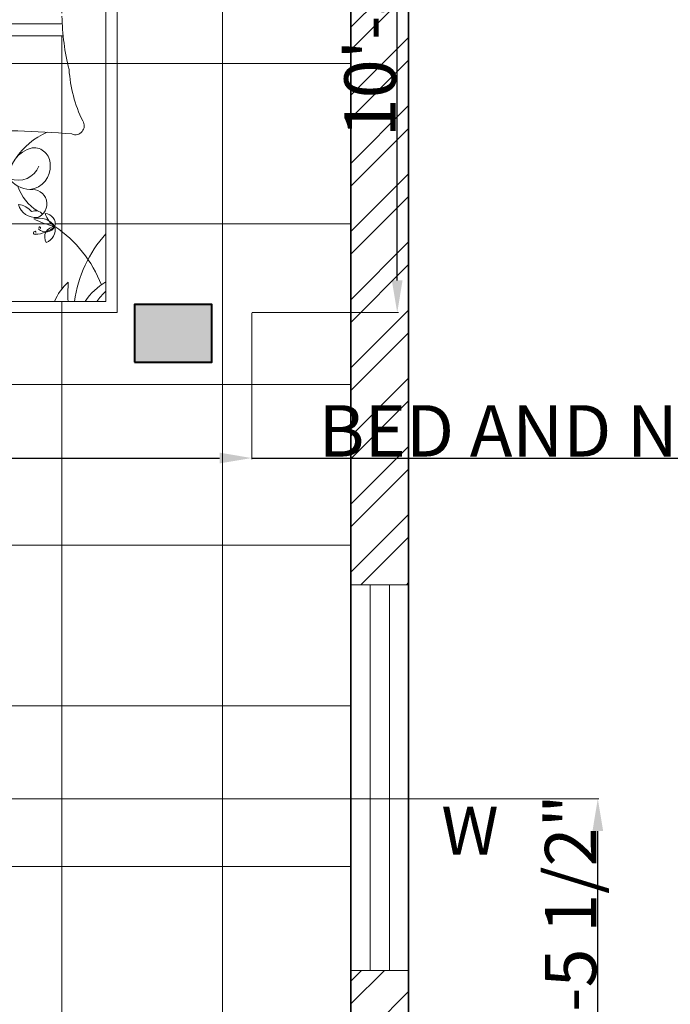
# Model space of a CAD drawing. Units: inches. Extents: x 351 to 1738, y -265 to 286.
# Tile 35 of 38: x 1506 to 1607, y -35 to 118. Entities that reach past the tile are written whole.
import ezdxf

# ---------------------------------------------------------------- set-up
doc = ezdxf.new("R2010")
doc.units = ezdxf.units.IN
doc.header["$MEASUREMENT"] = 0
for name, color, linetype, lineweight in [('A-ANNO-DIMS', 2, 'Continuous', 18), ('A-ANNO-SYMB', 7, 'Continuous', 18), ('A-COLS', 7, 'Continuous', 40), ('A-COLS-PATT', 6, 'Continuous', 13), ('A-FLOR-PATT', 9, 'Continuous', 9), ('A-FURN', 18, 'Continuous', 13), ('A-GLAZ', 4, 'Continuous', 18), ('A-WALL', 7, 'Continuous', 35), ('A-WALL-PATT', 152, 'Continuous', 13)]:
    doc.layers.add(name, color=color, linetype=linetype, lineweight=lineweight)
doc.styles.add('Annotative', font='arial.ttf')
doc.styles.get("Standard").update_dxf_attribs({"font": 'arial.ttf'})
doc.dimstyles.get("Standard").update_dxf_attribs({"dimtxt": 8, "dimasz": 5, "dimexe": 0.18, "dimexo": 0.0625, "dimgap": 0.09, "dimtad": 1, "dimtoh": 1, "dimzin": 0, "dimdsep": 46, "dimlunit": 4, "dimtxsty": 'Standard', "dimcen": 0, "dimclre": 256, "dimadec": 0, "dimazin": 0, "dimtfac": 1, "dimtofl": 0, "dimtmove": 0, "dimatfit": 3, "dimfxl": 1, "dimtolj": 1, "dimtzin": 0, "dimlwe": -1, "dimarcsym": 0})

# ---------------------------------------------------------------- blocks, each defined once
blk = doc.blocks.new('BED-DOUBLE-W-NIGHTSTANDS')
for p, q in [((121.41, 44.95), (28.44, 44.95)), ((121.55, 43.07), (28.44, 43.07))]:
    blk.add_line(p, q)
for points in [[(121.56, 54.36), (129.93, 54.36), (129.93, 0), (19.92, 0), (19.92, 54.36), (28.45, 54.36)], [(28.45, 52.61), (21.67, 52.61), (21.67, 1.75), (128.18, 1.75), (128.18, 52.61), (121.53, 52.61)]]:
    blk.add_lwpolyline(points)
blk.add_lwpolyline([(121.36, 46.14, 0.056112), (122.46, 37.83, 0.095341), (124.58, 29.84)], format="xyb")
for centre, radius, start, end in [((123.44, 29.07), 1.38, 246.5219, 33.8264), ((110.71, -118.52), 146.84, 85.2402, 91.8035), ((123.63, 17.62), 11.42, 113.6453, 146.3329), ((117.76, 21.21), 4.54, 103.079, 184.7067), ((116.98, 23.1), 2.55, 358.9462, 95.5144), ((115.93, 22.74), 3.61, 277.1143, 5.0551), ((114.52, 24.1), 3.5, 248.5779, 338.4181), ((116.56, 23.54), 4.38, 215.9599, 267.6409), ((121.25, 21.91), 7.12, 198.2955, 238.7386), ((116.76, 16.92), 2.26, 289.1312, 99.736), ((117.31, 17.61), 2.83, 195.6955, 274.031), ((114.26, 13.85), 3.01, 38.4175, 83.8338), ((117.23, 14.47), 1.39, 36.7319, 116.0245), ((122.02, 16.28), 3.37, 194.7031, 238.6173), ((118.68, 13.79), 1.63, 346.272, 87.0484), ((117.74, 11.59), 3.12, 35.7657, 104.5347), ((123.26, 26.86), 13.79, 242.8176, 257.4827), ((117.16, 12.42), 0.245, 78.5166, 272.0648), ((116.99, 17.16), 4.98, 272.0648, 311.1598), ((117.18, 12.55), 0.119, 322.0591, 78.5166), ((118.84, 14.16), 1.61, 226.2238, 332.3173), ((117.9, 13.23), 0.128, 290.2667, 226.2271), ((120.32, 11.76), 1.65, 91.7131, 211.5367), ((118.13, 12.94), 2.19, 290.9613, 12.2885), ((109.14, -2.86), 19.71, 21.4092, 55.6135), ((142.85, -0.91), 19.71, 138.1144, 172.255), ((127.59, -1.32), 8.01, 131.0454, 157.4453), ((149.54, 2.98), 27.26, 176.3481, 182.5919), ((132.97, -3.55), 9.6, 119.8884, 146.5383), ((136.42, -5.34), 11.97, 133.5186, 143.6964)]:
    blk.add_arc(centre, radius, start, end)
blk = doc.blocks.new('COL-9x12')
blk.add_lwpolyline([(0, 12), (0, 0), (9, 0), (9, 12)], close=True)
blk = doc.blocks.new('WIN-60')
for p, q in [((0, 6), (60, 6)), ((0, 3), (60, 3))]:
    blk.add_line(p, q)
blk.add_lwpolyline([(60, 0), (60, 9), (0, 9), (0, 0)], close=True)
blk = doc.blocks.new('*D46')
at = {"layer": 'A-ANNO-DIMS', "transparency": 16777216}
for p, q in [((1391.39, 72.13), (1391.39, 49.37)), ((1542.29, 72.13), (1542.29, 49.37))]:
    blk.add_line(p, q, dxfattribs=at)
at = {"layer": 'A-ANNO-DIMS', "color": 0, "lineweight": -2, "transparency": 16777216}
for p, q in [((1396.39, 49.55), (1537.29, 49.55)), ((1542.29, 49.55), (1738.09, 49.55))]:
    blk.add_line(p, q, dxfattribs=at)
at = {"layer": 'A-ANNO-DIMS', "color": 0, "transparency": 16777216}
for points in [[(1396.39, 50.39), (1396.39, 48.72), (1391.39, 49.55)], [(1537.29, 50.39), (1537.29, 48.72), (1542.29, 49.55)]]:
    blk.add_solid(points, dxfattribs=at)
at = {"layer": 'Defpoints', "color": 0, "transparency": 16777216}
for p in [(1391.39, 72.19), (1542.29, 72.19), (1542.29, 49.55)]:
    blk.add_point(p, dxfattribs=at)
at = {"layer": 'A-ANNO-DIMS', "color": 0, "transparency": 16777216, "insert": (1642.69, 53.78), "char_height": 8, "attachment_point": 5}
blk.add_mtext('\\A1;BED AND NIGHTSTANDS 12\'-7" TYP.', dxfattribs=at)
blk = doc.blocks.new('*D47')
at = {"layer": 'A-ANNO-DIMS', "transparency": 16777216}
for p, q in [((1542.36, 200.52), (1565.11, 200.52)), ((1542.36, 72.19), (1565.11, 72.19))]:
    blk.add_line(p, q, dxfattribs=at)
at = {"layer": 'A-ANNO-DIMS', "color": 0, "lineweight": -2, "transparency": 16777216}
blk.add_line((1564.93, 77.19), (1564.93, 195.52), dxfattribs=at)
at = {"layer": 'A-ANNO-DIMS', "color": 0, "transparency": 16777216}
for points in [[(1564.1, 195.52), (1565.76, 195.52), (1564.93, 200.52)], [(1564.1, 77.19), (1565.76, 77.19), (1564.93, 72.19)]]:
    blk.add_solid(points, dxfattribs=at)
at = {"layer": 'Defpoints', "color": 0, "transparency": 16777216}
for p in [(1542.29, 200.52), (1564.93, 200.52), (1542.29, 72.19)]:
    blk.add_point(p, dxfattribs=at)
at = {"layer": 'A-ANNO-DIMS', "color": 0, "transparency": 16777216, "insert": (1560.7, 136.35), "char_height": 8, "attachment_point": 5, "rotation": 90}
blk.add_mtext('\\A1;10\'-8 1/2" TYP.', dxfattribs=at)
blk = doc.blocks.new('*D66')
at = {"layer": 'A-ANNO-DIMS', "transparency": 16777216}
for p, q in [((1384.27, -3.5), (1596.33, -3.5)), ((1384.27, -45), (1596.33, -45))]:
    blk.add_line(p, q, dxfattribs=at)
at = {"layer": 'A-ANNO-DIMS', "color": 0, "lineweight": -2, "transparency": 16777216}
blk.add_line((1596.15, -40), (1596.15, -8.5), dxfattribs=at)
at = {"layer": 'A-ANNO-DIMS', "color": 0, "transparency": 16777216}
for points in [[(1595.32, -8.5), (1596.99, -8.5), (1596.15, -3.5)], [(1595.32, -40), (1596.99, -40), (1596.15, -45)]]:
    blk.add_solid(points, dxfattribs=at)
at = {"layer": 'Defpoints', "color": 0, "transparency": 16777216}
for p in [(1384.2, -3.5), (1596.15, -3.5), (1384.2, -45)]:
    blk.add_point(p, dxfattribs=at)
at = {"layer": 'A-ANNO-DIMS', "color": 0, "transparency": 16777216, "insert": (1591.92, -24.25), "char_height": 8, "attachment_point": 5, "rotation": 90}
blk.add_mtext('\\A1;3\'-5 1/2"', dxfattribs=at)

msp = doc.modelspace()

# ---------------------------------------------------------------- hatches: boundary and pattern name
at = {"layer": 'A-COLS-PATT'}
h = msp.add_hatch(color=256, dxfattribs=at)
h.dxf.hatch_style = 1
h.paths.add_polyline_path([(1112.704, 237.963), (1103.704, 237.963), (1103.704, 228.963), (1112.704, 228.963)])
h.paths.add_polyline_path([(1115.704, 237.963), (1112.704, 237.963), (1112.704, 228.963), (1115.704, 228.963)])
h.paths.add_polyline_path([(1043.704, 255.963), (1034.704, 255.963), (1034.704, 243.963), (1043.704, 243.963)])
h.paths.add_polyline_path([(1043.704, 210.963), (1034.704, 210.963), (1034.704, 198.963), (1043.704, 198.963)])
h.paths.add_polyline_path([(1043.704, -45.037), (1034.704, -45.037), (1034.704, -57.037), (1043.704, -57.037)])
h.paths.add_polyline_path([(1112.704, -45.037), (1103.704, -45.037), (1103.704, -57.037), (1112.704, -57.037)])
h.paths.add_polyline_path([(1112.704, -161.037), (1103.704, -161.037), (1103.704, -164.037), (1103.704, -173.037), (1112.704, -173.037)])
h.paths.add_polyline_path([(1043.704, -161.037), (1034.704, -161.037), (1034.704, -173.037), (1043.704, -173.037)])
h.paths.add_polyline_path([(1248.549, -164.037), (1236.549, -164.037), (1236.549, -173.037), (1248.549, -173.037)])
h.paths.add_polyline_path([(1248.549, -50), (1236.549, -50), (1236.549, -59), (1248.549, -59)])
h.paths.add_polyline_path([(1248.704, 73.463), (1244.704, 73.463), (1244.704, 64.463), (1248.704, 64.463)])
h.paths.add_polyline_path([(1244.704, 73.463), (1236.704, 73.463), (1236.704, 64.463), (1244.704, 64.463)])
h.paths.add_polyline_path([(1248.704, 237.963), (1236.704, 237.963), (1236.704, 228.963), (1248.704, 228.963)])
h.paths.add_polyline_path([(1392.204, 237.963), (1380.204, 237.963), (1380.204, 228.963), (1392.204, 228.963)])
h.paths.add_polyline_path([(1536.064, 237.963), (1524.064, 237.963), (1524.064, 228.963), (1536.064, 228.963)])
h.paths.add_polyline_path([(1536.064, 73.463), (1524.064, 73.463), (1524.064, 64.463), (1536.064, 64.463)])
h.paths.add_polyline_path([(1384.204, 73.463), (1380.204, 73.463), (1380.204, 64.463), (1384.204, 64.463)])
h.paths.add_polyline_path([(1392.064, 73.463), (1384.204, 73.463), (1384.204, 64.463), (1392.064, 64.463)])
h.paths.add_polyline_path([(1536.064, -53.037), (1524.064, -53.037), (1524.064, -57.037), (1536.064, -57.037)])
h.paths.add_polyline_path([(1536.064, -48.037), (1524.064, -48.037), (1524.064, -53.037), (1536.064, -53.037)])
h.paths.add_polyline_path([(1392.064, -48.037), (1380.064, -48.037), (1380.064, -56.5), (1380.065, -57.037), (1392.064, -57.037)])
h.paths.add_polyline_path([(1536.064, -164.037), (1524.064, -164.037), (1524.064, -173.037), (1536.064, -173.037)])
at = {"layer": 'A-FLOR-PATT', "transparency": 33554559}
h = msp.add_hatch(dxfattribs=at)
h.set_pattern_fill('ANSI37', color=256, scale=200, angle=135)
h.set_pattern_definition([(180, (1112.704, -164.037), (-2e-15, -25), []), (270, (1112.704, -164.037), (25, -5e-15), [])])
h.paths.add_polyline_path([(1380.064, 73.463), (1380.132, 148.463), (1338.064, 148.463), (1290.704, 148.463), (1290.704, 88.463), (1248.704, 88.463), (1248.704, -2.009), (1244.704, -2.009), (1244.704, 142.457), (1160.704, 142.457), (1160.704, 158.963), (1160.704, 170.137), (1160.704, 206.137), (1160.704, 228.963), (1112.704, 228.963), (1112.704, 209.963), (1112.704, 168.963), (1124.704, 168.963), (1124.704, 162.963), (1112.704, 162.963), (1112.704, 64.463), (1112.704, 60.463), (1112.704, 0.463), (1112.704, -48.026), (1146.804, -47.981), (1146.804, -35.691), (1207.804, -35.691), (1207.804, -47.902), (1236.542, -47.864), (1236.544, -50.009), (1248.5, -50.009), (1248.506, -102.915), (1248.512, -150.915), (1248.514, -164.037), (1248.549, -164.037), (1273.017, -164.037), (1273.017, -128.799), (1355.24, -128.799), (1355.24, -164.037), (1384.204, -164.037), (1384.204, -57.037), (1380.064, -57.037), (1380.064, -48.037), (1392.064, -48.037), (1392.064, -53.037), (1406.549, -53.037), (1406.549, -57.037), (1401.204, -57.037), (1401.204, -147.037), (1468.204, -147.037), (1468.204, -138.5), (1472.204, -138.5), (1472.204, -102.5), (1468.204, -102.5), (1468.204, -57.037), (1442.549, -57.037), (1442.549, -53.037), (1463.049, -53.037), (1463.049, -40.747), (1524.049, -40.747), (1524.049, -48.037), (1536.064, -48.037), (1536.064, -53.037), (1557.704, -53.037), (1557.704, 204.963), (1384.204, 204.963), (1384.204, 73.463), (1392.064, 73.463), (1392.064, 64.463), (1384.204, 64.463), (1384.204, -3.5), (1380.204, -3.537), (1380.204, 64.463), (1380.064, 64.463)])
h.paths.add_polyline_path([(1510.714, 86.458, -0.1039845), (1511.661, 85.595, 0.4704384), (1510.158, 87.614, 0.0961001)], flags=16)
h.paths.add_polyline_path([(1510.443, 100.266, 0.009798), (1504.693, 100.48, 0.0287898), (1504.6, 99.767, -0.1653311), (1505.519, 96.135, -0.1436014)], flags=16)
h.paths.add_polyline_path([(1487.201, 85.595, -0.1039845), (1488.148, 86.458, 0.0961001), (1488.704, 87.614, 0.4704384)], flags=0)
h.paths.add_polyline_path([(1495.052, 100.43), (1494.178, 100.43, -0.0264629), (1494.262, 99.774, -0.1442193)], flags=16)
h.paths.add_polyline_path([(1444.485, 86.458, -0.1039845), (1445.433, 85.595, 0.4704384), (1443.93, 87.614, 0.0961001)], flags=16)
h.paths.add_polyline_path([(1420.972, 85.595, -0.1039845), (1421.92, 86.458, 0.0961001), (1422.475, 87.614, 0.4704384)], flags=16)
h.paths.add_polyline_path([(1428.632, 100.335, 0.0010541), (1427.971, 100.309, -0.0215241), (1428.033, 99.774, -0.1143008)], flags=16)
h.paths.add_polyline_path([(1419.906, 143.708, 0.0249793), (1420.222, 157.526), (1421.573, 159.101), (1421.573, 175.369), (1391.393, 175.369), (1391.393, 200.519), (1542.294, 200.519), (1542.294, 175.369), (1512.028, 175.369, 0.0198653), (1511.521, 153.838, 0.0251335), (1512.758, 118.323, 0.0205529), (1512.942, 115.253), (1419.834, 115.253, -0.0004142), (1419.843, 124.798), (1413.059, 124.798), (1413.059, 84.437, -0.0618528), (1415.831, 80.45, -0.0930773), (1420.972, 85.595, -0.2675367), (1422.371, 84.732, 0.0851103), (1424.052, 84.616, -0.8853927), (1424.033, 84.851, -1.1258145), (1424.073, 84.366, -0.0879871), (1422.371, 84.732, -0.2675367), (1422.326, 83.089, -0.3705421), (1420.972, 85.595, 0.0930773), (1415.831, 80.45, -0.0874142), (1417.914, 73.937), (1418.941, 73.937, 0.0272504), (1418.913, 76.906, -0.1157032), (1421.051, 73.937), (1445.354, 73.937, -0.1157032), (1447.492, 76.906, 0.0272504), (1447.464, 73.937), (1448.491, 73.937, -0.0874142), (1450.574, 80.45, 0.0930773), (1445.433, 85.595, -0.3705421), (1444.079, 83.089, -0.2675367), (1444.034, 84.732, -0.0879871), (1442.332, 84.366, -1.1258145), (1442.372, 84.851, -2.0327363), (1442.364, 84.368, 0.0863779), (1444.034, 84.732, -0.2675367), (1445.433, 85.595, -0.0930773), (1450.574, 80.45, -0.2577317), (1466.483, 90.927, -0.4786702), (1468.832, 91.907, -0.4786702), (1471.18, 90.927, -0.26264), (1483.053, 81.78, -0.0718662), (1487.201, 85.595, -0.2675367), (1488.6, 84.732, 0.0851103), (1490.28, 84.616, -0.8853927), (1490.262, 84.851, -1.1258145), (1490.301, 84.366, -0.0879871), (1488.6, 84.732, -0.2675367), (1488.554, 83.089, -0.3705421), (1487.201, 85.595, 0.0718662), (1483.053, 81.78, -0.1320648), (1484.143, 73.937), (1485.169, 73.937, 0.0272504), (1485.142, 76.906, -0.1157032), (1487.28, 73.937), (1511.582, 73.937, -0.1157032), (1513.72, 76.906, 0.0272504), (1513.693, 73.937), (1514.719, 73.937, -0.0874142), (1516.802, 80.45, 0.0930773), (1511.661, 85.595, -0.3705421), (1510.308, 83.089, -0.2675367), (1510.262, 84.732, -0.0879871), (1508.561, 84.366, -1.1258145), (1508.601, 84.851, -2.0327363), (1508.592, 84.368, 0.0863779), (1510.262, 84.732, -0.2675367), (1511.661, 85.595, -0.0930773), (1516.802, 80.45, -0.0618528), (1519.575, 84.437), (1519.575, 73.937), (1413.059, 73.937), (1413.059, 124.798), (1419.843, 124.798, -0.0008205)], flags=16)
h.paths.add_polyline_path([(1220.149, 54.133, -0.1039845), (1220.869, 53.476, 0.4704384), (1219.727, 55.011, 0.0961001)], flags=16)
h.paths.add_polyline_path([(1219.944, 64.626, 0.009798), (1215.574, 64.789, 0.0287898), (1215.503, 64.247, -0.1653311), (1216.201, 61.487, -0.1436014)], flags=16)
h.paths.add_polyline_path([(1209.779, 64.449, 0.0974459), (1209.339, 64.751), (1208.247, 64.751, 0.1273905), (1207.7, 64.326, 0.1715858), (1206.95, 61.475, -0.1588542), (1207.636, 59.45, 0.0158984), (1207.795, 59.218, 0.0615457), (1208.598, 59.616, 0.1754158), (1208.638, 60.099, -0.2847793), (1209.348, 62.472, 0.3262165)], flags=16)
h.paths.add_polyline_path([(1169.818, 54.133, -0.1039845), (1170.538, 53.476, 0.4704384), (1169.396, 55.011, 0.0961001)], flags=16)
h.paths.add_polyline_path([(1159.017, 62.472, 0.2847642), (1158.307, 60.099, -0.1754332), (1158.267, 59.616, 0.3929302), (1159.448, 64.449, -0.3262298)], flags=16)
h.paths.add_polyline_path([(1156.342, 58.239, -0.1783213), (1154.011, 55.31, -0.1747359), (1154.722, 55.233, -0.2008015), (1156.27, 56.086, 0.1269899), (1157.283, 58.991, -0.0912053)], flags=16)
h.paths.add_polyline_path([(1156.624, 61.413, 0.1572752), (1157.316, 64.247, 0.1696217)], flags=16)
h.paths.add_polyline_path([(1152.67, 54.133, -0.0961001), (1151.95, 53.476, 0.0640762), (1154.465, 54.384, 0.1990158)], flags=16)
h.paths.add_polyline_path([(1202.281, 53.476, -0.1039845), (1203, 54.133, 0.0961001), (1203.423, 55.011, 0.4704384)], flags=0)
h.paths.add_polyline_path([(1151.139, 97.64, 0.0249793), (1151.379, 108.141), (1152.406, 109.338), (1152.406, 121.701), (1129.47, 121.701), (1129.47, 140.814), (1244.149, 140.814), (1244.149, 121.701), (1221.148, 121.701, 0.0198653), (1220.763, 105.338, 0.0251335), (1221.703, 78.349, 0.0205529), (1221.843, 76.016), (1151.078, 76.016, -0.1287433), (1148.786, 65.037, 0.5393525), (1150.327, 64.171, -0.027594), (1163.481, 64.751, 0.0976954), (1163.04, 64.449, 0.3262165), (1163.471, 62.472, -0.2847765), (1164.181, 60.099, -0.1947567), (1165.846, 61.443, -0.1554021), (1165.172, 64.247, -0.1660224), (1165.869, 61.475, -0.1770142), (1167.852, 62.77, -0.4482027), (1169.974, 60.807, -0.3934987), (1167.679, 57.86, -0.8955483), (1168.438, 54.524, -0.3557668), (1166.218, 56.086, -0.066024), (1165.505, 57.539), (1165.251, 56.243, -0.3717324), (1164.02, 59.758, -0.3736141), (1163.04, 64.449, -0.0976954), (1163.481, 64.751, 0.0213538), (1153.294, 64.429, -0.1341826), (1156.695, 61.368, 0.1868727), (1154.636, 62.77, 0.4482027), (1152.514, 60.807, 0.4037263), (1154.905, 57.846, 0.7112192), (1153.334, 55, 0.5315397), (1151.95, 53.476, -0.2675367), (1153.013, 52.821, 0.0851103), (1154.29, 52.732, -0.8853927), (1154.276, 52.911, -1.1258145), (1154.306, 52.543, -0.0879871), (1153.013, 52.821, -0.2675367), (1152.978, 51.572, -0.3705421), (1151.95, 53.476, 0.0930773), (1148.043, 49.566, -0.0874142), (1149.626, 44.617), (1150.406, 44.617, 0.0272504), (1150.385, 46.873, -0.1157032), (1152.01, 44.617), (1170.478, 44.617, -0.1157032), (1172.103, 46.873, 0.0272504), (1172.082, 44.617), (1172.862, 44.617, -0.0874142), (1174.445, 49.566, 0.0930773), (1170.538, 53.476, -0.3705421), (1169.51, 51.572, -0.2675367), (1169.475, 52.821, -0.0879871), (1168.182, 52.543, -1.1258145), (1168.212, 52.911, -2.0327363), (1168.206, 52.544, 0.0863779), (1169.475, 52.821, -0.2675367), (1170.538, 53.476, -0.0930773), (1174.445, 49.566, -0.2577317), (1186.536, 57.528, -0.4786702), (1188.321, 58.273, -0.4786702), (1190.106, 57.528, -0.26264), (1199.128, 50.577, -0.0718662), (1202.281, 53.476, -0.2675367), (1203.344, 52.821, 0.0851103), (1204.621, 52.732, -0.8853927), (1204.607, 52.911, -1.1258145), (1204.637, 52.543, -0.0879871), (1203.344, 52.821, -0.2675367), (1203.309, 51.572, -0.3705421), (1202.281, 53.476, 0.0718662), (1199.128, 50.577, -0.1320648), (1199.957, 44.617), (1200.737, 44.617, 0.0272504), (1200.716, 46.873, -0.1157032), (1202.341, 44.617), (1220.809, 44.617, -0.1157032), (1222.434, 46.873, 0.0272504), (1222.413, 44.617), (1223.193, 44.617, -0.0874142), (1224.776, 49.566, 0.0930773), (1220.869, 53.476, -0.3705421), (1219.841, 51.572, -0.2675367), (1219.806, 52.821, -0.0879871), (1218.513, 52.543, -1.1258145), (1218.543, 52.911, -2.0327363), (1218.537, 52.544, 0.0863779), (1219.806, 52.821, -0.2675367), (1220.869, 53.476, -0.0930773), (1224.776, 49.566, -0.0618528), (1226.883, 52.597), (1226.883, 44.617), (1145.936, 44.617), (1145.936, 83.269), (1151.091, 83.269, -0.0008205)], flags=16)
h.paths.add_polyline_path([(1218.01, 57.86, -0.8955483), (1218.769, 54.524, -0.3557668), (1216.549, 56.086, -0.066024), (1215.836, 57.539), (1215.582, 56.243, -0.3717324), (1214.351, 59.758, -0.3736141), (1213.371, 64.449, 0.3262165), (1213.802, 62.472, -0.2847765), (1214.512, 60.099, -0.1947567), (1216.177, 61.443, -0.1799907), (1218.183, 62.77, -0.4482027), (1220.305, 60.807, -0.3934987)], flags=16)
h.paths.add_polyline_path([(1424.735, 91.363, -0.3934987), (1421.715, 95.241, -0.4482027), (1424.507, 97.824, -0.1799907), (1427.147, 96.077, -0.1947567), (1429.338, 94.309, -0.2847765), (1430.272, 97.432, 0.3262165), (1430.839, 100.034, -0.3736141), (1429.55, 93.861, -0.3717324), (1427.929, 89.235), (1427.596, 90.941, -0.066024), (1426.657, 89.029, -0.3557668), (1423.736, 86.973, -0.8955483)], flags=16)
h.paths.add_polyline_path([(1238.033, 131.257, -1), (1227.329, 131.257, -1)], flags=0)
h.paths.add_polyline_path([(1235.357, 131.257, -1), (1230.005, 131.257, -1)], flags=0)
h.paths.add_polyline_path([(1214.039, 54.243, 0.1543819), (1214.38, 53.992, 0.3589549), (1213.613, 54.016, 0.6039484), (1214.379, 53.657, 0.3713191), (1213.968, 52.872, 0.1879935), (1214.312, 52.809, -0.592455), (1213.953, 52.967, -0.2942791), (1214.083, 53.691, -1.3001871), (1213.881, 54.134, -0.2837621), (1214.469, 53.896, 1.1509396)], flags=16)
h.paths.add_polyline_path([(1212.091, 56.286, -0.4084338), (1211.337, 56.445, -0.0362594), (1211.098, 56.848, -0.2360976), (1211.59, 56.63, 0.0353445), (1211.835, 56.543, -0.4752408), (1212.091, 56.286, -0.4752408), (1212.438, 56.182, 0.0353445), (1212.631, 56.007, -0.2360976), (1213.056, 55.676, -0.0362594), (1212.588, 55.697, -0.4084338)], flags=16)
h.paths.add_polyline_path([(1211.469, 50.297, 0.296043), (1210.47, 50.527, 0.310883), (1211.931, 50.148, 0.0212546)], flags=16)
h.paths.add_polyline_path([(1213.739, 51.818, -0.0362594), (1213.271, 51.838, -0.4084337), (1212.774, 52.427, -0.0947856), (1212.293, 50.703, 1.1504738), (1212.911, 50.232, 0.1662877), (1213.265, 50.68, -0.0252543), (1212.603, 50.13, 1.0879317), (1212.471, 49.407, 0.1662877), (1213.02, 49.251, -0.016128), (1212.567, 49.563, -0.286859), (1212.217, 49.638, 0.0221563), (1212.046, 50.055, -0.6461302), (1212.185, 50.498, 0.0884116), (1212.732, 52.077, -1.1860374), (1213.121, 52.323, 0.0353445), (1213.314, 52.148, -0.2360976)], flags=16)
h.paths.add_polyline_path([(1212.094, 50.342, -0.0485241), (1211.54, 49.605, -1.1038339), (1211.397, 48.738, -0.7855147), (1211.683, 48.254, -0.3920429), (1210.948, 48.525, -0.3928194), (1210.561, 47.995, -0.592455), (1210.201, 48.153, -0.2942791), (1210.331, 48.877, -0.7041716), (1210.316, 49.592, -0.6793441), (1210.729, 50.112, 0.5636764)], flags=16)
h.paths.add_polyline_path([(1211.274, 49.829, -0.1398258), (1210.745, 49.859, -0.2178785), (1210.948, 49.509, -0.4985724)], flags=0)
h.paths.add_polyline_path([(1433.426, 81.49, -0.181571), (1434.245, 81.788, -0.0080665), (1433.726, 82.205, 0.0455784), (1432.755, 81.242, 0.1790113)], flags=16)
h.paths.add_polyline_path([(1434.146, 81.009, -0.1324418), (1433.645, 80.771, 0.2590893), (1433.234, 80.471, -0.1802109), (1433.392, 80.805, -0.1699398), (1432.758, 81.109, 0.0326525), (1433.273, 80.474, -0.4933627), (1434.046, 80.146, -0.3904966)], flags=16)
h.paths.add_polyline_path([(1434.83, 80.047, -0.9475376), (1435.294, 79.576, -0.2991282), (1434.625, 79.404, -0.2704392), (1435.01, 78.591, -0.592455), (1434.537, 78.382, -0.3928194), (1434.027, 79.08, -0.3920429), (1433.06, 78.723, -0.3520423), (1433.003, 79.197, -0.1972159), (1433.75, 79.734, -0.7136405), (1434.447, 79.939, -0.2147903), (1434.819, 80.475, 0.4088333), (1435.075, 80.803, -0.2261519)], flags=16)
h.paths.add_polyline_path([(1432.67, 81.217, -0.4542182), (1431.897, 79.923, -0.4144105), (1431.301, 80.035, 0.0161291), (1431.897, 80.445, 0.2795702), (1432.073, 80.871, -0.2895037), (1431.103, 81.321, -0.4144105), (1430.978, 81.915, 0.0161296), (1431.586, 81.521, 0.341293), (1432.125, 81.583, -0.8131856)], flags=16)
h.paths.add_polyline_path([(1429.893, 86.381, -0.9475376), (1430.358, 85.91, -0.1731062), (1429.984, 85.712, -0.0388172), (1431.625, 84.214, -0.0879005), (1432.097, 88.549, -0.0497684), (1431.254, 88.49, -0.2360976), (1431.814, 88.925, 0.0353445), (1432.067, 89.155, -0.4752408), (1432.524, 89.291, -0.4752408), (1432.86, 89.63, 0.0353445), (1433.182, 89.744, -0.2360976), (1433.83, 90.032, -0.0362594), (1433.516, 89.502, -0.4084338), (1432.524, 89.291, -0.3124239), (1432.106, 88.58, 0.0885594), (1431.625, 84.214, -0.4084337), (1430.971, 83.439, -0.0362594), (1430.355, 83.412, -0.2360976), (1430.914, 83.847, 0.0353445), (1431.168, 84.078, -0.4752408), (1431.625, 84.214, 0.0388172), (1429.984, 85.712, -0.3217316), (1429.333, 86.048, -0.32743), (1429.883, 86.809, 0.4088333), (1430.138, 87.138, -0.2261519)], flags=16)
h.paths.add_polyline_path([(1211.206, 58.616, -0.9997836), (1211.336, 59.323, -0.6149935)], flags=16)
h.paths.add_polyline_path([(1210.288, 49.429, 0.1543819), (1210.629, 49.178, 0.3589549), (1209.861, 49.202, 0.6039484), (1210.627, 48.843, -0.5348247), (1210.806, 49.295, 0.7483464)], flags=16)
h.paths.add_polyline_path([(1209.589, 51.828, -0.0087906), (1209.775, 51.753, 0.1122315), (1209.466, 52.019, 1.4188509), (1209.014, 51.708, -0.4587257), (1208.651, 51.073, -0.592455), (1208.291, 51.232, -0.2942791), (1208.421, 51.955, -1.3001871), (1208.219, 52.398, -0.2260052), (1208.719, 52.257, -0.4755189), (1209.158, 52.369, -1.4554994), (1209.603, 52.664, 0.4213049), (1209.191, 52.262, -0.5912116), (1208.979, 51.796, 0.4973986), (1209.773, 51.333, 0.6493116)], flags=16)
h.paths.add_polyline_path([(1208.029, 52.041, 0.5446671), (1208.832, 52.045, 0.220132)], flags=0)
h.paths.add_polyline_path([(1210.438, 51.425, -0.2041997), (1210.277, 52.018, 0.2708262), (1209.915, 52.897, 0.3241145)], flags=0)
h.paths.add_polyline_path([(1209.668, 52.407, -0.60139), (1208.99, 52.221, -0.3949159), (1208.248, 52.83, -0.8367916), (1208.651, 53.017, -0.3384876), (1209.039, 52.571, 0.1941379), (1209.191, 52.262, 0.4139945), (1209.712, 52.475, 0.5177103), (1210.503, 51.416, 0.401922), (1209.493, 50.93, 0.2063956), (1209.516, 50.165, -0.3194629), (1210.417, 51.418, -0.466635)], flags=16)
h.paths.add_polyline_path([(1206.601, 56.086, -0.3557668), (1204.381, 54.524, -0.9211983), (1205.236, 57.846, 0.2065693), (1207.614, 58.991, -0.1269899)], flags=16)
h.paths.add_polyline_path([(1435.487, 82.816, 0.5277653), (1436.615, 83.361, 0.5085402), (1437.05, 82.433, 0.592455), (1437.524, 82.641, 0.3312448), (1436.963, 83.548, 0.3878632), (1437.808, 83.626, 0.5929544), (1437.618, 84.176, 0.2260158), (1436.961, 83.99, 0.3182053), (1437.588, 84.854, 0.6893744), (1437.05, 84.991, 0.3357648), (1436.539, 84.41, -0.1569934), (1436.404, 84.065, -0.4346112), (1436.961, 83.99, -0.2147903), (1437.333, 84.526, 0.4088333), (1437.588, 84.854, -0.2261519), (1437.343, 84.097, -0.9475376), (1437.808, 83.626, -0.2991282), (1437.139, 83.455, -0.2704392), (1437.524, 82.641, -0.592455), (1437.05, 82.433, -0.3928194), (1436.541, 83.13, -0.4396601), (1435.475, 82.794, -0.174614), (1435.942, 82.244, -0.2063956), (1435.912, 81.237, -0.2708262), (1435.125, 82.208, 0.2079765), (1434.686, 82.904, -0.1964955)], flags=16)
h.paths.add_polyline_path([(1435.386, 84.832, 0.270811), (1434.91, 83.676, -0.2042174), (1434.699, 82.895, 0.3241145)], flags=0)
h.paths.add_polyline_path([(1435.68, 84.18, -0.2176564), (1435.554, 83.304, -0.1767045), (1436.236, 83.778, -0.3730364)], flags=0)
h.paths.add_polyline_path([(1435.566, 100.034, 0.3262165), (1436.133, 97.432, -0.2847765), (1437.067, 94.309, -0.1947567), (1439.258, 96.077, -0.1554021), (1438.371, 99.767, -0.1660224), (1439.289, 96.12, -0.1770142), (1441.897, 97.824, -0.4482027), (1444.69, 95.241, -0.3934987), (1441.67, 91.363, -0.8955483), (1442.669, 86.973, -0.3557668), (1439.748, 89.029, -0.066024), (1438.809, 90.941), (1438.476, 89.235, -0.3717324), (1436.855, 93.861, -0.3736141)], flags=16)
h.paths.add_polyline_path([(1191.252, 49.507, -0.2740221), (1190.658, 48.409, 0.2675367), (1191.311, 47.344, 0.3705421)], flags=0)
h.paths.add_polyline_path([(1190.301, 49.717, 0.1990158), (1188.619, 49.04, 0.0640762), (1191.252, 49.507, -0.0961001)], flags=0)
h.paths.add_polyline_path([(1189.518, 47.857, 1.1258145), (1189.676, 47.523, 2.0446052)], flags=0)
h.paths.add_polyline_path([(1464.974, 80.372, 0.2740221), (1465.756, 78.927, -0.0830131)], flags=0)
h.paths.add_polyline_path([(1464.974, 80.372, 0.3705421), (1464.897, 77.525, 0.5763244)], flags=0)
h.paths.add_polyline_path([(1464.974, 80.372, -0.4704384), (1467.284, 81.372, -0.0961001), (1466.226, 80.648, -0.1990158), (1468.439, 79.757, -0.0640762)], flags=0)
h.paths.add_polyline_path([(1189.511, 56.43, -0.2594668), (1188.321, 56.391, -0.2594668), (1187.13, 56.43, 0.0851103), (1188.193, 55.716, -0.8853927), (1188.27, 55.878, -1.1960133), (1188.355, 55.442, 0.1014587)], flags=0)
h.paths.add_polyline_path([(1188.321, 57.596, 0.0780722), (1187.678, 57.24, 0.0155503), (1188.321, 57.136, 0.0155503), (1188.964, 57.24, 0.0780722)], flags=0)
h.paths.add_polyline_path([(1190.164, 55.365, -0.5763244), (1190.106, 57.528, -0.1982945), (1188.321, 58.319, -0.1982945), (1186.536, 57.528, -0.5763244), (1186.477, 55.365, -0.3705421), (1186.536, 57.528, 0.1982945), (1188.321, 58.319, 0.1982945), (1190.106, 57.528, -0.3705421)], flags=0)
h.paths.add_polyline_path([(1188.372, 55.878, 1.1258145), (1188.529, 55.544, 2.0446052)], flags=0)
h.paths.add_polyline_path([(1186.341, 49.717, -0.0961001), (1185.389, 49.507, 0.0640762), (1188.022, 49.04, 0.1990158)], flags=0)
h.paths.add_polyline_path([(1185.389, 49.507, -0.2675367), (1185.984, 48.409, 0.0851103), (1187.046, 47.695, -0.8853927), (1187.123, 47.857, -1.1258145), (1186.966, 47.523, -0.0879871), (1185.984, 48.409, -0.2675367), (1185.331, 47.344, -0.3705421)], flags=0)
h.paths.add_polyline_path([(1399.441, 187.944, -1), (1413.525, 187.944, -1)], flags=0)
h.paths.add_polyline_path([(1402.962, 187.944, -1), (1410.004, 187.944, -1)], flags=0)
h.paths.add_polyline_path([(1357.663, -72.245), (1377.272, -72.245), (1377.272, -91.854), (1357.663, -91.854)], flags=16)
h.paths.add_polyline_path([(1467.256, 78.201, -1.1258145), (1467.049, 77.761, -2.0446052)], flags=0)
h.paths.add_polyline_path([(1468.822, 88.714, 0.9411249), (1469.106, 88.316, 1.1371523), (1468.765, 88.755, 0.890986), (1468.99, 88.245, 0.0948283), (1470.398, 89.481, -0.2675367), (1471.18, 90.927, -0.0281232), (1469.678, 90.547, -0.0287737), (1469.948, 90.311, -0.0203267), (1468.832, 90.41, -0.0203267), (1467.716, 90.311, -0.0287737), (1467.986, 90.547, -0.0281232), (1466.483, 90.927, -0.2675367), (1467.265, 89.481, 0.0851103), (1468.663, 88.542, -1.2023159)], flags=0)
h.paths.add_polyline_path([(1178.25, 124.523, -0.1199286), (1165.65, 124.145, -0.1073492), (1159.133, 124.446, -0.1028906), (1159.132, 130.465, -0.0748968), (1158.993, 137.956, 0.002027), (1167.844, 137.479, -0.07553), (1180.337, 137.666, -0.0758613), (1186.502, 137.688, -0.1409896), (1186.272, 130.046, -0.0954805), (1186.729, 124.748, -0.10603)], flags=0)
h.paths.add_polyline_path([(1469.225, 79.757, -0.1990158), (1471.437, 80.648, -0.0961001), (1470.379, 81.372, -0.4704384), (1472.689, 80.372, -0.3705421), (1472.766, 77.525, -0.2675367), (1471.907, 78.927, -0.0879863), (1470.615, 77.761, -1.1258491), (1470.408, 78.201, -2.0327363), (1470.642, 77.778, 0.0863779), (1471.907, 78.927, -0.2675367), (1472.689, 80.372, -0.0640762)], flags=0)
h.paths.add_polyline_path([(1430.423, 186.902, -0.0748968), (1430.24, 196.758, 0.002027), (1441.887, 196.131, -0.07553), (1458.326, 196.377, -0.0758613), (1466.438, 196.406, -0.1409896), (1466.136, 186.35, -0.0954805), (1466.737, 179.378, -0.10603), (1455.58, 179.082, -0.1199286), (1439, 178.585, -0.1073492), (1430.425, 178.981, -0.1028906)], flags=0)
h.paths.add_polyline_path([(1162.258, 49.939, 0.3357645), (1161.87, 49.497, -0.1569936), (1161.767, 49.235, -0.4346112), (1162.19, 49.178, -0.2147903), (1162.473, 49.585, 1.5291948)], flags=16)
h.paths.add_polyline_path([(1161.683, 49.021, 0.5815181), (1161.268, 49.583, 0.5927609)], flags=16)
h.paths.add_polyline_path([(1162.602, 48.058, 0.3713191), (1162.192, 48.843, 0.4345332), (1162.88, 48.962, 0.1850806), (1162.197, 48.926, 1.1218369)], flags=16)
h.paths.add_polyline_path([(1161.443, 48.941, -1.3071038), (1161.495, 48.571, -0.2177521), (1161.136, 48.254, 0.6973029), (1161.871, 49.048, 0.1215141)], flags=16)
h.paths.add_polyline_path([(1162.531, 49.429, -0.2070837), (1162.05, 49.146, -0.9920299)], flags=16)
h.paths.add_polyline_path([(1161.304, 49.578, -0.7196675), (1161.513, 50.079, -0.1304275), (1160.836, 50.168, 0.0395926)], flags=0)
h.paths.add_polyline_path([(1162.036, 50.584, -0.0080665), (1161.642, 50.9, 0.0293675), (1161.35, 50.297, -0.2057884)], flags=16)
h.paths.add_polyline_path([(1162.882, 51.392, -0.1247327), (1162.763, 51.828, -0.1011907), (1162.399, 51.438, -0.153425)], flags=0)
h.paths.add_polyline_path([(1164.235, 51.85, -0.3091075), (1164.513, 51.136, -0.6271245), (1163.781, 51.603, -0.6859091), (1162.777, 51.219, -0.2332851), (1163.303, 50.165, -0.2708262), (1162.705, 50.903, 0.2041997), (1162.381, 51.425, 0.204182), (1162.542, 52.018, -0.2708414), (1162.903, 52.897, -0.1272607), (1163.219, 52.529, -1.1686811), (1163.781, 52.587, -0.3291117), (1164.168, 53.017, -0.8367917), (1164.571, 52.83, -0.1933406), (1164.391, 52.338, -0.9475376), (1164.744, 51.981, -0.2991282)], flags=16)
h.paths.add_polyline_path([(1163.598, 51.937, -1.2629561), (1163.236, 51.831, 0.0125754), (1162.971, 51.721, 0.2306566), (1163.151, 52.407, -0.1648982), (1163.178, 52.661, -0.4493201), (1163.628, 52.262, -0.721477), (1164.154, 52.088, -0.8499982)], flags=0)
h.paths.add_polyline_path([(1161.613, 58.616, -0.9804131), (1161.525, 59.049, -2.9089348)], flags=16)
h.paths.add_polyline_path([(1160.252, 49.166, -0.4144105), (1159.799, 49.251, 0.0161291), (1160.252, 49.563, 0.2795702), (1160.386, 49.887, -0.2895037), (1159.649, 50.229, -0.4144105), (1159.554, 50.68, 0.0161296), (1160.015, 50.381, 0.6178854), (1160.526, 50.703, -0.0947856), (1160.045, 52.427, -0.1404436), (1159.682, 52.042, -0.0578559), (1159.3, 51.872, 0.5448433), (1160.046, 52.419, -0.0881216), (1160.404, 55.721, -0.0497684), (1159.763, 55.676, -0.2360976), (1160.188, 56.007, 0.0353445), (1160.381, 56.182, -0.4752408), (1160.728, 56.286, -0.4752408), (1160.984, 56.543, 0.0353445), (1161.229, 56.63, -0.2360976), (1161.721, 56.848, -0.0362594), (1161.482, 56.445, -0.4084338), (1160.728, 56.286, -0.3124239), (1160.411, 55.745, 0.0885594), (1160.045, 52.427, 0.1070813), (1160.634, 50.498, -0.4947977), (1160.839, 50.149, -0.4542182)], flags=16)
h.paths.add_polyline_path([(1160.666, 49.808, -2.0765276), (1160.828, 50.172, 0.0195861)], flags=0)
h.paths.add_polyline_path([(1158.439, 53.992, 0.1543819), (1158.78, 54.243, 0.7483463), (1158.262, 54.109, -0.3382251), (1158.492, 53.839, -0.1708158), (1159.124, 53.779, 0.4957286), (1158.938, 54.134, 0.2260157)], flags=16)
h.paths.add_polyline_path([(1160.045, 52.427, 0.0388172), (1158.798, 53.565, -0.1198178), (1158.574, 53.586, -0.3091075), (1158.851, 52.872, -0.1879935), (1158.506, 52.809, 0.592455), (1158.866, 52.967, 0.3312448), (1158.44, 53.657, 0.2012451), (1158.798, 53.565, -0.034023), (1159.901, 52.578, -0.0442527), (1159.698, 52.323, -0.4752408)], flags=16)
h.paths.add_polyline_path([(1336.926, -95.392), (1336.926, -117.945), (1291.82, -117.945), (1291.82, -95.392)], flags=16)
h.paths.add_polyline_path([(1357.535, -97.244), (1357.726, -96.697, 0.0348443)], flags=16)
h.paths.add_polyline_path([(1376.693, -96.478), (1377.301, -96.5, 0.0314968), (1375.907, -96.424), (1357.726, -96.424)], flags=16)
h.paths.add_polyline_path([(1379.403, -119.667, 0.0267056), (1380.043, -119.439, -0.0152991)], flags=16)
h.paths.add_polyline_path([(1357.726, -120.202), (1357.821, -120.202), (1357.821, -120.201)], flags=16)
h.paths.add_polyline_path([(1354.171, -104.592), (1354.469, -98.672, 0.0111377)], flags=16)
h.paths.add_polyline_path([(1355.058, -119.136), (1354.578, -118.539, 0.1431635)], flags=16)
h.paths.add_polyline_path([(1378.851, -96.821), (1378.85, -96.82), (1378.85, -96.82, -0.0496798), (1380.055, -97.191), (1378.85, -96.82, 0.1500541), (1375.135, -97.188), (1375.136, -119.44, -0.0099698), (1374.747, -116.649), (1357.726, -116.649, 0.1693849), (1357.535, -119.382), (1357.535, -119.382), (1357.535, -119.382, 0.0348176), (1357.726, -119.928), (1357.726, -119.928), (1357.726, -119.929, -0.0348772), (1357.535, -119.382), (1355.507, -119.382), (1355.317, -119.278), (1357.535, -119.382, -0.1693939), (1357.726, -116.649, -0.0391513), (1374.686, -116.113, -0.0020149), (1374.625, -115.546, 0.1153223), (1369.915, -115.474, 0.0609215), (1369.922, -101.154, 0.1151459), (1374.625, -101.079, -0.0020164), (1374.686, -100.513, -0.0391511), (1357.726, -99.977), (1374.747, -99.977, -0.0099633), (1375.135, -97.188), (1375.135, -97.188, -0.1501081)], flags=16)
h.paths.add_polyline_path([(1490.963, 91.363, -0.3934987), (1487.944, 95.241, -0.4482027), (1490.736, 97.824, -0.1799907), (1493.376, 96.077, -0.1947567), (1495.567, 94.309, -0.2847765), (1496.501, 97.432, 0.3262165), (1497.068, 100.034, -0.3736141), (1495.778, 93.861, -0.3717324), (1494.158, 89.235), (1493.824, 90.941, -0.066024), (1492.886, 89.029, -0.3557668), (1489.964, 86.973, -0.8955483)], flags=16)
h.paths.add_polyline_path([(1354.86, -97.658), (1355.316, -97.348, 0.1019112)], flags=16)
h.paths.add_polyline_path([(1497.063, 83.327, 0.1767244), (1496.37, 83.785, -0.4051388), (1496.016, 83.384, 0.4973986), (1497.06, 82.774, 0.6493116), (1496.818, 83.426, -0.0087906)], flags=16)
h.paths.add_polyline_path([(1496.339, 83.783, 0.5927609), (1496.886, 84.522, 0.5815181)], flags=16)
h.paths.add_polyline_path([(1495.11, 82.641, 0.592455), (1495.583, 82.433, 0.6769152), (1495.805, 83.59, 0.3756693)], flags=16)
h.paths.add_polyline_path([(1495.015, 84.176, -0.145057), (1495.301, 84.526, -0.4088333), (1495.045, 84.854, 0.2206292), (1495.381, 84.152, -0.199594), (1495.851, 83.764, -0.5240172), (1494.826, 83.626, -0.5929976)], flags=16)
h.paths.add_polyline_path([(1501.655, 81.915, -0.0161291), (1501.048, 81.521, -0.3927187), (1500.462, 81.37, -0.2106699), (1500.607, 81.142, 0.3066994)], flags=16)
h.paths.add_polyline_path([(1500.11, 89.291, -0.4084338), (1499.118, 89.502, -0.0362594), (1498.803, 90.032, -0.2360976), (1499.451, 89.744, 0.0353445), (1499.774, 89.63, -0.4752408), (1500.11, 89.291, -0.4752408), (1500.567, 89.155, 0.0353445), (1500.82, 88.925, -0.2360976), (1501.379, 88.49, -0.0362594), (1500.763, 88.516, -0.4084338)], flags=16)
h.paths.add_polyline_path([(1498.908, 82.205, -0.0513217), (1500.013, 81.134, -0.5879306), (1500.234, 81.676, 0.1070813), (1501.009, 84.214, -0.03529)], flags=16)
h.paths.add_polyline_path([(1496.93, 83.875, -0.2063956), (1497.247, 84.832, -0.2708262), (1497.724, 83.676, 0.2079765), (1497.944, 82.884, -0.3814554)], flags=16)
h.paths.add_polyline_path([(1496.721, 81.237, 0.2708125), (1497.509, 82.208, -0.2042157), (1497.935, 82.895, 0.3241145)], flags=16)
h.paths.add_polyline_path([(1497.529, 80.125, -0.145057), (1497.814, 80.475, -0.703182), (1498.282, 81.178, -0.1229248), (1497.977, 81.714, -0.2708368), (1499.207, 81.49, 0.2079641), (1499.993, 81.248, -0.2651454), (1499.278, 80.472, 0.3819006), (1498.808, 79.947, -0.3059049), (1498.848, 79.519, 0.4994816), (1498.574, 79.217, -0.4587257), (1498.097, 78.382, -0.592455), (1497.624, 78.591, -0.2704392), (1498.009, 79.404, -0.299116), (1497.34, 79.576, -0.5930157)], flags=16)
h.paths.add_polyline_path([(1500.736, 79.923, 0.4144105), (1501.333, 80.035, -0.3216484), (1500.192, 80.765, 0.0198856), (1499.976, 81.251, 0.4653307)], flags=16)
h.paths.add_polyline_path([(1501.009, 84.214, -0.0388172), (1502.649, 85.712, -0.1730946), (1502.276, 85.91, -0.5930157), (1502.465, 86.46, -0.145057), (1502.751, 86.809, -0.4088333), (1502.495, 87.138, 0.2206292), (1502.831, 86.436, -0.199594), (1503.301, 86.048, -0.3217316), (1502.649, 85.712, 0.0388172), (1501.009, 84.214, 0.1224486), (1501.412, 83.755, 0.4754908), (1501.335, 84.226, 0.055822), (1501.719, 83.847, -0.2360976), (1502.278, 83.412, -0.0362594), (1501.663, 83.439, -0.4084338)], flags=16)
h.paths.add_polyline_path([(1501.794, 100.034, 0.3262165), (1502.362, 97.432, -0.2847765), (1503.295, 94.309, -0.1947567), (1505.486, 96.077, -0.1799907), (1508.126, 97.824, -0.4482027), (1510.918, 95.241, -0.3934987), (1507.899, 91.363, -0.8955483), (1508.898, 86.973, -0.3557668), (1505.976, 89.029, -0.066024), (1505.038, 90.941), (1504.704, 89.235, -0.3717324), (1503.084, 93.861, -0.3736141)], flags=16)
h.paths.add_polyline_path([(1146.29, 131.257, -1), (1135.587, 131.257, -1)], flags=0)
h.paths.add_polyline_path([(1143.614, 131.257, -1), (1138.262, 131.257, -1)], flags=0)
h.paths.add_polyline_path([(1524.064, 73.463), (1536.064, 73.463), (1536.064, 64.463), (1524.064, 64.463)], flags=16)
h.paths.add_polyline_path([(1520.162, 187.944, -1), (1534.246, 187.944, -1)], flags=0)
h.paths.add_polyline_path([(1530.725, 187.944), (1527.204, 187.944), (1527.204, 184.423, 0.4142136)], flags=0)
h.paths.add_polyline_path([(1278.415, -91.154), (1331.067, -91.154), (1331.067, -80.583), (1278.415, -80.583)], flags=24)
h.paths.add_polyline_path([(1266.655, -79.354), (1354.738, -79.354), (1354.738, -67.817), (1266.655, -67.817)], flags=24)
h.paths.add_polyline_path([(1115.482, 206.184), (1155.098, 206.184), (1155.098, 217.714), (1115.482, 217.714)], flags=24)
h.paths.add_polyline_path([(1161.771, 8.501), (1222.466, 8.501), (1222.466, 19.079), (1161.771, 19.079)], flags=24)
h.paths.add_polyline_path([(1164.656, 18.795), (1210.615, 18.795), (1210.615, 30.324), (1164.656, 30.324)], flags=24)
h.paths.add_polyline_path([(1368.147, -32.882), (1379.362, -32.882), (1379.362, -21.733), (1368.147, -21.733)], flags=24)
h.paths.add_polyline_path([(1244.842, -31.012), (1256.057, -31.012), (1256.057, -19.863), (1244.842, -19.863)], flags=24)
h.paths.add_polyline_path([(1114.589, 195.739), (1156.517, 195.739), (1156.517, 206.31), (1114.589, 206.31)], flags=24)
h.paths.add_polyline_path([(1436.398, 37.632), (1505.131, 37.632), (1505.131, 48.203), (1436.398, 48.203)], flags=24)
h.paths.add_polyline_path([(1435.991, 47.919), (1507.906, 47.919), (1507.906, 59.456), (1435.991, 59.456)], flags=24)
h.paths.add_polyline_path([(1415.107, -124.896), (1457.038, -124.896), (1457.038, -114.318), (1415.107, -114.318)], flags=24)
h.paths.add_polyline_path([(1417.992, -114.602), (1457.609, -114.602), (1457.609, -103.073), (1417.992, -103.073)], flags=24)
at = {"layer": 'A-WALL-PATT'}
h = msp.add_hatch(dxfattribs=at)
h.set_pattern_fill('ANSI32', color=256, scale=20)
h.set_pattern_definition([(45, (1034.704, -173.037), (-5.3033, 5.3033), []), (45, (1038.24, -173.037), (-5.3033, 5.3033), [])])
h.paths.add_polyline_path([(1043.704, -57.037), (1034.704, -57.037), (1034.704, -81.037), (1043.704, -81.037)])
h.paths.add_polyline_path([(1043.704, 198.963), (1034.704, 198.963), (1034.704, -45.037), (1043.704, -45.037)])
h.paths.add_polyline_path([(1043.704, 243.963), (1034.704, 243.963), (1034.704, 237.963), (1034.704, 210.963), (1043.704, 210.963)])
h.paths.add_polyline_path([(1112.704, 255.963), (1043.704, 255.963), (1043.704, 246.963), (1103.704, 246.963), (1103.704, 237.963), (1112.704, 237.963), (1112.704, 251.963)])
h.paths.add_polyline_path([(1056.704, 207.963), (1043.704, 207.963), (1043.704, 198.963), (1056.704, 198.963)])
h.paths.add_polyline_path([(1103.704, 207.963), (1092.704, 207.963), (1092.704, 198.963), (1103.704, 198.963)])
h.paths.add_polyline_path([(1112.704, 228.963), (1103.704, 228.963), (1103.704, 74.963), (1112.704, 74.963), (1112.704, 97.5)])
h.paths.add_polyline_path([(1284.129, -164.037), (1248.549, -164.037), (1248.549, -173.037), (1284.129, -173.037)])
h.paths.add_polyline_path([(1524.064, -164.037), (1472.204, -164.037), (1472.204, -138.5), (1468.204, -138.5), (1468.204, -164.037), (1344.129, -164.037), (1344.129, -173.037), (1524.064, -173.037)])
h.paths.add_polyline_path([(1384.204, -57.037), (1380.065, -57.037), (1380.204, -164.037), (1384.204, -164.037)])
h.paths.add_polyline_path([(1566.704, -138), (1557.704, -138), (1557.704, -164.037), (1536.064, -164.037), (1536.064, -173.037), (1566.704, -173.037)])
h.paths.add_polyline_path([(1566.704, -30.189), (1557.704, -30.189), (1557.704, -53.037), (1536.064, -53.037), (1536.064, -57.037), (1557.704, -57.037), (1557.704, -102), (1566.704, -102)])
h.paths.add_polyline_path([(1524.064, -53.037), (1442.549, -53.037), (1442.549, -57.037), (1468.204, -57.037), (1468.204, -102.5), (1472.204, -102.5), (1472.204, -57.037), (1524.064, -57.037)])
h.paths.add_polyline_path([(1566.704, 120.993), (1557.704, 120.993), (1557.704, 29.811), (1566.704, 29.811)])
h.paths.add_polyline_path([(1384.204, 64.463), (1380.204, 64.463), (1380.204, -3.5), (1384.204, -3.5)])
h.paths.add_polyline_path([(1266.549, 237.963), (1248.704, 237.963), (1248.704, 228.963), (1266.549, 228.963)])
h.paths.add_polyline_path([(1329.549, 237.963), (1302.549, 237.963), (1302.549, 228.963), (1329.549, 228.963)])
h.paths.add_polyline_path([(1380.204, 237.963), (1365.549, 237.963), (1365.549, 228.963), (1380.204, 228.963)])
h.paths.add_polyline_path([(1524.064, 237.963), (1392.204, 237.963), (1392.204, 228.963), (1524.064, 228.963)])
h.paths.add_polyline_path([(1384.204, 228.963), (1380.204, 228.963), (1380.204, 73.463), (1384.204, 73.463)])
h.paths.add_polyline_path([(1566.704, 237.963), (1536.064, 237.963), (1536.064, 228.963), (1557.704, 228.963), (1557.704, 180.993), (1566.704, 180.993)])

# ---------------------------------------------------------------- linework, layer by layer
at = {"layer": 'A-WALL'}
for p, q in [((1566.704, -173.037), (1566.704, 237.963)), ((1557.704, -53.037), (1557.704, 228.963))]:
    msp.add_line(p, q, dxfattribs=at)

# ---------------------------------------------------------------- block references
at = {"layer": 'A-COLS', "rotation": 90.00000000000082}
msp.add_blockref('COL-9x12', (1536.064, 64.462), dxfattribs=at)
at = {"layer": 'A-FURN'}
msp.add_blockref('BED-DOUBLE-W-NIGHTSTANDS', (1391.393, 72.188), dxfattribs=at)
at = {"layer": 'A-GLAZ', "rotation": 90.00000000000003}
msp.add_blockref('WIN-60', (1566.704, -30.189), dxfattribs=at)

# ---------------------------------------------------------------- texts
at = {"layer": 'A-ANNO-SYMB', "style": 'Annotative'}
msp.add_text('W', height=7.433, dxfattribs=at).set_placement((1571.805, -12.157))

# ---------------------------------------------------------------- dimensions: what is measured, and where the dimension line sits
at = {"layer": 'A-ANNO-DIMS'}
dim = msp.add_linear_dim(base=(1564.929, 200.519), p1=(1542.294, 72.188), p2=(1542.294, 200.519), angle=90, text='<> TYP.', dimstyle='Standard', override={"dimdec": 1, "dimlfac": 1, "dimrnd": 0, "dimzin": 1, "dimdsep": 46, "dimlunit": 4, "dimfrac": 2}, dxfattribs=at)
dim.commit()
dim.dimension.update_dxf_attribs({"geometry": '*D47', "text_midpoint": (1560.702, 136.353)})
dim = msp.add_linear_dim(base=(1542.294, 49.553), p1=(1391.393, 72.188), p2=(1542.294, 72.188), text='BED AND NIGHTSTANDS <> TYP.', dimstyle='Standard', override={"dimdec": 1, "dimlfac": 1, "dimrnd": 0, "dimzin": 1, "dimdsep": 46, "dimlunit": 4, "dimfrac": 2}, dxfattribs=at)
dim.commit()
dim.dimension.update_dxf_attribs({"geometry": '*D46', "text_midpoint": (1642.691, 53.779)})
dim = msp.add_linear_dim(base=(1596.154, -3.5), p1=(1384.204, -45), p2=(1384.204, -3.5), angle=90, dimstyle='Standard', override={"dimdec": 1, "dimlfac": 1, "dimrnd": 0, "dimzin": 1, "dimdsep": 46, "dimlunit": 4, "dimfrac": 2}, dxfattribs=at)
dim.commit()
dim.dimension.update_dxf_attribs({"geometry": '*D66', "text_midpoint": (1591.925, -24.25)})

doc.saveas('drawing.dxf')
